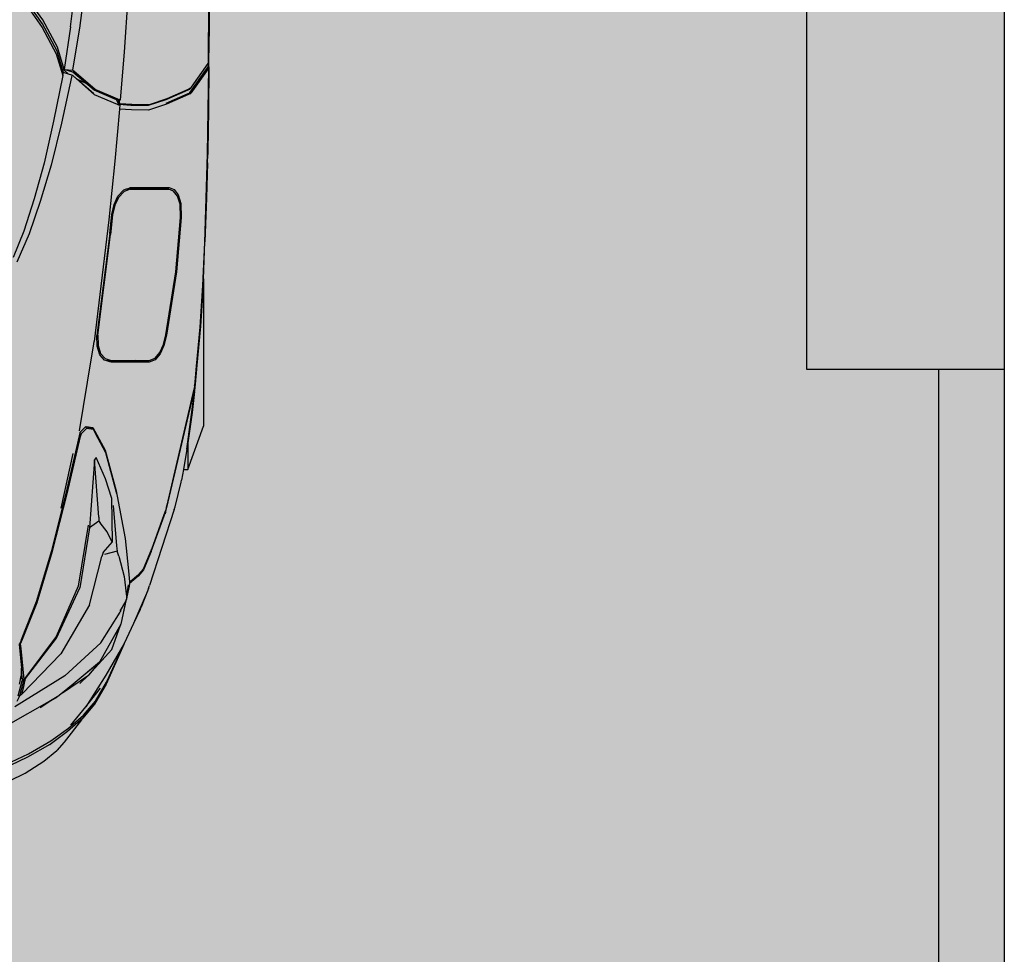
# Model space of a CAD drawing. Units: inches. Extents: x 1884 to 2398, y 474 to 1488.
# Tile 22 of 39: x 2352 to 2397, y 577 to 620. Entities that reach past the tile are written whole.
import ezdxf

# ---------------------------------------------------------------- set-up
doc = ezdxf.new("R2010")
doc.units = ezdxf.units.IN
doc.header["$MEASUREMENT"] = 0
doc.layers.get('0').update_dxf_attribs({"color": 250})
for name, color, linetype, lineweight in [('A-ANNO-DIMS', 2, 'Continuous', 18), ('A-WALL-PATT', 250, 'Continuous', 13), ('C-PROP', 7, 'Continuous', 30), ('C-VEHI', 8, 'Continuous', 18)]:
    doc.layers.add(name, color=color, linetype=linetype, lineweight=lineweight)
doc.layers.add('Edges', color=250, linetype='Continuous')
doc.layers.add('L-PVMT-PATT', color=9, linetype='Continuous', lineweight=13, true_color=0xc7c8ca)
doc.styles.get("Standard").update_dxf_attribs({"font": 'arial.ttf'})
doc.dimstyles.get("Standard").update_dxf_attribs({"dimtxt": 7, "dimasz": 0.18, "dimexe": 0.18, "dimexo": 0.0625, "dimgap": 0.09, "dimtad": 0, "dimtih": 1, "dimtoh": 1, "dimzin": 0, "dimdsep": 46, "dimlunit": 3, "dimtxsty": 'Standard', "dimcen": 0.09, "dimadec": 0, "dimazin": 0, "dimtfac": 1, "dimtofl": 0, "dimtmove": 0, "dimatfit": 3, "dimfxl": 1, "dimtolj": 1, "dimtzin": 0, "dimarcsym": 0})

# ---------------------------------------------------------------- blocks, each defined once
blk = doc.blocks.new('Nissan Qashqai pl')
at = {"layer": 'Edges'}
for p, q in [((10.6151, 12.8159), (10.6644, 12.8162)), ((10.6176, 12.8164), (10.6651, 12.8167)), ((10.6644, 12.8162), (10.7078, 12.8159)), ((10.6651, 12.8167), (10.666, 12.8167)), ((10.666, 12.8167), (10.677, 12.8167)), ((10.6729, 12.8157), (10.7082, 12.8156)), ((10.6809, 12.8167), (10.677, 12.8167)), ((10.7128, 12.8166), (10.6809, 12.8167)), ((10.7078, 12.8159), (10.7083, 12.8156)), ((10.7082, 12.8156), (10.7078, 12.8159)), ((10.7085, 12.8153), (10.7082, 12.8156)), ((10.7082, 12.8156), (10.7083, 12.8156)), ((10.7083, 12.8156), (10.7087, 12.8153)), ((10.7083, 12.8156), (10.7125, 12.8156)), ((10.7087, 12.8153), (10.7363, 12.7959)), ((10.7139, 12.8164), (10.7125, 12.8156)), ((10.7137, 12.8148), (10.7125, 12.8156)), ((10.7128, 12.8166), (10.7625, 12.8161)), ((10.7128, 12.8166), (10.724, 12.8166)), ((10.7137, 12.8148), (10.7138, 12.8147)), ((10.7418, 12.7947), (10.7138, 12.8147)), ((10.7139, 12.8164), (10.7148, 12.8157)), ((10.7628, 12.8158), (10.7139, 12.8164)), ((10.7148, 12.8157), (10.7429, 12.7956)), ((10.7685, 12.8161), (10.724, 12.8166)), ((10.7625, 12.8161), (10.7628, 12.8161)), ((10.7628, 12.8161), (10.8099, 12.8152)), ((10.8131, 12.8149), (10.7628, 12.8158)), ((10.7688, 12.8161), (10.7685, 12.8161)), ((10.8099, 12.8152), (10.7688, 12.8161)), ((10.8099, 12.8152), (10.8131, 12.8152)), ((10.8134, 12.8152), (10.8131, 12.8152)), ((10.8644, 12.8135), (10.8131, 12.8149)), ((10.8134, 12.8152), (10.8142, 12.8152)), ((10.8142, 12.8152), (10.8142, 12.8152)), ((10.8237, 12.8149), (10.8142, 12.8152)), ((10.8237, 12.8149), (10.864, 12.8138)), ((10.8596, 12.8138), (10.8589, 12.8138)), ((10.8642, 12.8136), (10.8596, 12.8138)), ((10.864, 12.8138), (10.8642, 12.8138)), ((10.8642, 12.8138), (10.9152, 12.812)), ((10.9158, 12.8118), (10.8644, 12.8135)), ((10.9577, 12.8101), (10.9152, 12.812)), ((10.9657, 12.8095), (10.9158, 12.8118)), ((10.9577, 12.8101), (10.9649, 12.8097)), ((10.9577, 12.8101), (11.1283, 12.8101)), ((10.9649, 12.8097), (11.0127, 12.8067)), ((11.0138, 12.8064), (10.9657, 12.8095)), ((11.0127, 12.8067), (11.0576, 12.8026)), ((11.1783, 12.7921), (11.1283, 12.8101)), ((10.7363, 12.7959), (10.7376, 12.795)), ((10.7432, 12.7954), (10.7426, 12.7954)), ((10.7429, 12.7956), (10.7432, 12.7954)), ((10.7441, 12.7954), (10.7432, 12.7954)), ((10.7432, 12.7954), (10.744, 12.7948)), ((11.059, 12.8023), (11.0138, 12.8064)), ((11.0576, 12.8026), (11.0798, 12.8008)), ((11.0768, 12.8008), (11.059, 12.8023)), ((11.0811, 12.8004), (11.0768, 12.8008)), ((11.0798, 12.8008), (11.0872, 12.7999)), ((11.0827, 12.8001), (11.0811, 12.8004)), ((11.0827, 12.8001), (11.0813, 12.7998)), ((11.0836, 12.8002), (11.0827, 12.8001)), ((11.0856, 12.7994), (11.0827, 12.8001)), ((11.0872, 12.7999), (11.0836, 12.8002)), ((11.0836, 12.8002), (11.0882, 12.7992)), ((11.2196, 12.7681), (11.0856, 12.7994)), ((11.0883, 12.7998), (11.0872, 12.7999)), ((11.0882, 12.7992), (11.2222, 12.7676)), ((11.0883, 12.7998), (11.1123, 12.797)), ((11.1147, 12.7965), (11.0883, 12.7998)), ((11.1123, 12.797), (11.1475, 12.7921)), ((11.1547, 12.791), (11.1147, 12.7965)), ((10.7387, 12.794), (10.7376, 12.795)), ((10.7376, 12.795), (10.7378, 12.7946)), ((10.7378, 12.7946), (10.7379, 12.7945)), ((10.7378, 12.7946), (10.7385, 12.7932)), ((10.7385, 12.7932), (10.7497, 12.7679)), ((10.7387, 12.794), (10.7396, 12.7922)), ((10.7396, 12.7922), (10.7507, 12.7669)), ((10.743, 12.7939), (10.7418, 12.7947)), ((10.7434, 12.793), (10.743, 12.7939)), ((10.7437, 12.7921), (10.7434, 12.793)), ((10.7438, 12.7921), (10.7437, 12.7921)), ((10.7438, 12.7921), (10.7549, 12.7666)), ((10.744, 12.7948), (10.7448, 12.793)), ((10.7448, 12.793), (10.7559, 12.7674)), ((10.8607, 12.7808), (10.8708, 12.7841)), ((10.8708, 12.7841), (10.8869, 12.7844)), ((10.8869, 12.7844), (10.9499, 12.7789)), ((11.1475, 12.7921), (11.1525, 12.7914)), ((11.1475, 12.7921), (11.1783, 12.7921)), ((11.1525, 12.7914), (11.1547, 12.791)), ((11.1547, 12.791), (11.1783, 12.787)), ((11.1783, 12.787), (11.1783, 12.7921)), ((11.1783, 12.787), (11.1906, 12.7849)), ((11.1906, 12.7849), (11.1909, 12.7849)), ((11.193, 12.7845), (11.1909, 12.7849)), ((11.2215, 12.7775), (11.193, 12.7845)), ((10.8523, 12.7704), (10.8546, 12.7762)), ((10.8565, 12.7757), (10.8543, 12.7702)), ((10.8546, 12.7762), (10.8607, 12.7808)), ((10.8622, 12.7801), (10.8565, 12.7757)), ((10.8716, 12.7832), (10.8622, 12.7801)), ((10.887, 12.7835), (10.8716, 12.7832)), ((10.9498, 12.7781), (10.887, 12.7835)), ((11.0226, 12.7668), (10.9498, 12.7781)), ((10.9499, 12.7789), (11.0229, 12.7676)), ((11.2247, 12.7764), (11.2215, 12.7775)), ((11.2247, 12.7764), (11.3124, 12.7479)), ((10.7497, 12.7679), (10.7565, 12.7473)), ((10.7507, 12.7669), (10.7575, 12.7462)), ((10.7559, 12.7674), (10.7626, 12.7467)), ((10.8523, 12.7255), (10.8523, 12.7704)), ((10.8543, 12.7702), (10.8538, 12.753)), ((10.8543, 12.7255), (10.8543, 12.7702)), ((11.0339, 12.7639), (11.0226, 12.7668)), ((11.0229, 12.7676), (11.0348, 12.7645)), ((11.0429, 12.7597), (11.0339, 12.7639)), ((11.0348, 12.7645), (11.0444, 12.7601)), ((11.2247, 12.767), (11.2163, 12.7689)), ((11.22, 12.768), (11.2196, 12.7681)), ((11.2247, 12.767), (11.22, 12.768)), ((11.2222, 12.7676), (11.2271, 12.7664)), ((11.2253, 12.7668), (11.2247, 12.767)), ((11.2304, 12.7649), (11.2253, 12.7668)), ((11.2253, 12.7668), (11.2271, 12.7664)), ((11.2271, 12.7664), (11.2296, 12.7658)), ((11.2271, 12.7664), (11.2277, 12.7662)), ((11.2277, 12.7662), (11.2296, 12.7658)), ((11.2732, 12.7496), (11.2277, 12.7662)), ((11.2704, 12.7504), (11.2304, 12.7649)), ((10.8528, 12.7503), (10.8535, 12.7521)), ((10.8528, 12.742), (10.8528, 12.7503)), ((10.8535, 12.7521), (10.8538, 12.753)), ((10.8538, 12.7521), (10.8535, 12.7521)), ((10.8538, 12.753), (10.8538, 12.7521)), ((10.8538, 12.7521), (10.8538, 12.7502)), ((10.8538, 12.7502), (10.8538, 12.742)), ((11.0497, 12.7542), (11.0429, 12.7597)), ((11.0444, 12.7601), (11.0516, 12.7542)), ((11.0523, 12.7475), (11.0497, 12.7542)), ((11.0516, 12.7542), (11.0543, 12.7473)), ((11.2702, 12.7507), (11.2704, 12.7504)), ((11.2704, 12.7506), (11.2707, 12.7503)), ((11.2707, 12.7503), (11.2704, 12.7504)), ((11.2719, 12.7498), (11.2707, 12.7503)), ((11.2934, 12.741), (11.2719, 12.7498)), ((10.7565, 12.7473), (10.7563, 12.7273)), ((10.7575, 12.7462), (10.7572, 12.7263)), ((10.7626, 12.7467), (10.7623, 12.7269)), ((10.8528, 12.742), (10.8538, 12.742)), ((10.8528, 12.7419), (10.8528, 12.742)), ((10.8538, 12.7419), (10.8528, 12.7419)), ((10.8528, 12.7242), (10.8528, 12.7419)), ((10.8538, 12.742), (10.8538, 12.7419)), ((10.8538, 12.7214), (10.8538, 12.7419)), ((11.0528, 12.73), (11.0523, 12.7475)), ((11.0523, 12.7312), (11.0523, 12.7475)), ((11.0543, 12.7473), (11.0543, 12.7035)), ((11.2732, 12.7496), (11.2946, 12.7409)), ((11.3, 12.735), (11.2934, 12.741)), ((11.2946, 12.7409), (11.3018, 12.7346)), ((11.3161, 12.7467), (11.3124, 12.7479)), ((11.3161, 12.7467), (11.3376, 12.7381)), ((11.3192, 12.7454), (11.3566, 12.7294)), ((10.7563, 12.7273), (10.7553, 12.7134)), ((11.0523, 12.7312), (11.0528, 12.73)), ((11.0523, 12.7287), (11.0523, 12.7312)), ((11.0528, 12.7274), (11.0523, 12.7287)), ((11.0523, 12.7037), (11.0523, 12.7287)), ((11.0528, 12.7274), (11.0528, 12.73)), ((11.0528, 12.73), (11.0538, 12.7273)), ((11.0528, 12.7274), (11.0528, 12.6985)), ((11.0538, 12.7273), (11.0538, 12.7018)), ((11.3081, 12.7253), (11.3, 12.735)), ((11.3018, 12.7346), (11.3103, 12.7249)), ((11.3405, 12.7369), (11.3376, 12.7381)), ((11.3405, 12.7369), (11.3566, 12.7294)), ((11.3566, 12.7294), (11.3796, 12.7187)), ((10.6318, 12.7228), (10.6955, 12.7184)), ((10.6955, 12.7184), (10.7509, 12.714)), ((10.7572, 12.7263), (10.7563, 12.7126)), ((10.7623, 12.7269), (10.7615, 12.7131)), ((10.8528, 12.7242), (10.8523, 12.7255)), ((10.8538, 12.7214), (10.8528, 12.7242)), ((10.855, 12.7181), (10.8538, 12.7214)), ((10.8543, 12.7255), (10.8569, 12.7184)), ((10.8622, 12.7114), (10.855, 12.7181)), ((10.8569, 12.7184), (10.8637, 12.712)), ((11.2091, 12.7103), (11.2583, 12.7196)), ((11.2583, 12.7196), (11.2956, 12.7234)), ((11.2787, 12.7123), (11.3022, 12.7186)), ((11.2956, 12.7234), (11.3085, 12.7247)), ((11.3022, 12.7186), (11.3252, 12.7213)), ((11.3086, 12.7247), (11.3081, 12.7253)), ((11.3081, 12.7253), (11.3087, 12.7247)), ((11.3085, 12.7247), (11.3086, 12.7247)), ((11.3086, 12.7247), (11.3087, 12.7247)), ((11.3087, 12.7247), (11.3103, 12.7249)), ((11.3103, 12.7249), (11.3103, 12.7249)), ((11.3103, 12.7249), (11.3106, 12.7249)), ((11.3106, 12.7249), (11.314, 12.7238)), ((11.317, 12.7227), (11.3119, 12.7236)), ((11.3132, 12.7243), (11.3256, 12.7215)), ((11.314, 12.7238), (11.317, 12.7227)), ((11.314, 12.7238), (11.3242, 12.7216)), ((11.3242, 12.7216), (11.317, 12.7227)), ((11.3198, 12.7211), (11.3252, 12.7213)), ((11.3242, 12.7216), (11.3256, 12.7215)), ((11.3252, 12.7213), (11.3283, 12.7214)), ((11.3256, 12.7215), (11.3283, 12.7214)), ((11.3283, 12.7214), (11.3297, 12.7206)), ((11.3297, 12.7206), (11.3446, 12.7173)), ((11.3297, 12.7206), (11.3302, 12.7203)), ((11.3302, 12.7203), (11.3446, 12.7173)), ((11.3302, 12.7203), (11.3394, 12.7152)), ((11.3446, 12.7173), (11.3571, 12.7146)), ((11.3796, 12.7187), (11.4164, 12.6974)), ((11.3796, 12.7187), (11.3807, 12.7182)), ((11.3807, 12.7182), (11.4267, 12.6979)), ((11.4228, 12.6989), (11.3807, 12.7182)), ((10.7501, 12.7114), (10.7387, 12.6849)), ((10.7507, 12.7098), (10.7397, 12.684)), ((10.7563, 12.7109), (10.7449, 12.6843)), ((10.7507, 12.7132), (10.7501, 12.7114)), ((10.7506, 12.7111), (10.7507, 12.7132)), ((10.7507, 12.7132), (10.7509, 12.714)), ((10.751, 12.7132), (10.7507, 12.7132)), ((10.7511, 12.7107), (10.7507, 12.7098)), ((10.7524, 12.7106), (10.7507, 12.7098)), ((10.7522, 12.7131), (10.7509, 12.714)), ((10.7516, 12.7131), (10.7509, 12.714)), ((10.7519, 12.7128), (10.7511, 12.7107)), ((10.7522, 12.7131), (10.7516, 12.7131)), ((10.7519, 12.7128), (10.7516, 12.7131)), ((10.7526, 12.7124), (10.7519, 12.7128)), ((10.7553, 12.7134), (10.7522, 12.7131)), ((10.7524, 12.7106), (10.7526, 12.7124)), ((10.7556, 12.7122), (10.7524, 12.7106)), ((10.7526, 12.7124), (10.7526, 12.7127)), ((10.7532, 12.712), (10.7526, 12.7124)), ((10.7556, 12.7122), (10.7532, 12.712)), ((10.7561, 12.7125), (10.7556, 12.7122)), ((10.7561, 12.7125), (10.7563, 12.7126)), ((10.7563, 12.7125), (10.7561, 12.7125)), ((10.7563, 12.7123), (10.7561, 12.7123)), ((10.7563, 12.7126), (10.7573, 12.7135)), ((10.7563, 12.7126), (10.7563, 12.7125)), ((10.7569, 12.7125), (10.7563, 12.7109)), ((10.7569, 12.7125), (10.7563, 12.7125)), ((10.7563, 12.7125), (10.7563, 12.7123)), ((10.7573, 12.7135), (10.7569, 12.7125)), ((10.7573, 12.7135), (10.7604, 12.7132)), ((10.7604, 12.7132), (10.7615, 12.7131)), ((10.7615, 12.7131), (10.8218, 12.7077)), ((10.8218, 12.7077), (10.8896, 12.7008)), ((10.8718, 12.7068), (10.8622, 12.7114)), ((10.8637, 12.712), (10.8727, 12.7077)), ((10.8836, 12.7041), (10.8718, 12.7068)), ((10.8727, 12.7077), (10.8839, 12.7051)), ((10.8839, 12.7051), (10.9067, 12.7029)), ((11.156, 12.6966), (11.203, 12.7093)), ((11.1589, 12.6971), (11.2062, 12.7098)), ((11.2121, 12.7043), (11.189, 12.6968)), ((11.203, 12.7093), (11.2091, 12.7103)), ((11.2062, 12.7098), (11.2091, 12.7103)), ((11.2622, 12.7051), (11.2121, 12.7043)), ((11.2199, 12.706), (11.2666, 12.7097)), ((11.2622, 12.7051), (11.2601, 12.7037)), ((11.2743, 12.6942), (11.2622, 12.7051)), ((11.2666, 12.7097), (11.2729, 12.7104)), ((11.2787, 12.7123), (11.2729, 12.7104)), ((11.2729, 12.7104), (11.2766, 12.6957)), ((11.3394, 12.7152), (11.3434, 12.7138)), ((11.3394, 12.7152), (11.342, 12.7137)), ((11.379, 12.6915), (11.3434, 12.7138)), ((11.3583, 12.7142), (11.3571, 12.7146)), ((11.3571, 12.7146), (11.3821, 12.7008)), ((11.3583, 12.7142), (11.3821, 12.7008)), ((11.3864, 12.7044), (11.3583, 12.7142)), ((11.4163, 12.6775), (11.3864, 12.7044)), ((10.9054, 12.702), (10.8836, 12.7041)), ((10.8896, 12.7008), (11.0304, 12.6838)), ((10.9054, 12.702), (11.0232, 12.6871)), ((11.0231, 12.6882), (10.9067, 12.7029)), ((11.0443, 12.6911), (11.0501, 12.6964)), ((11.052, 12.6958), (11.0458, 12.6903)), ((11.0501, 12.6964), (11.0523, 12.7037)), ((11.0528, 12.6985), (11.052, 12.6958)), ((11.0538, 12.7018), (11.0528, 12.6985)), ((11.0543, 12.7035), (11.0538, 12.7018)), ((11.1298, 12.6823), (11.156, 12.6966)), ((11.1365, 12.6851), (11.1589, 12.6971)), ((11.189, 12.6968), (11.1644, 12.6862)), ((11.2505, 12.6987), (11.2401, 12.6908)), ((11.2601, 12.7037), (11.2505, 12.6987)), ((11.2743, 12.6942), (11.2791, 12.6927)), ((11.3821, 12.7008), (11.4014, 12.69)), ((11.4164, 12.6974), (11.4531, 12.6744)), ((11.4243, 12.6982), (11.4228, 12.6989)), ((11.4464, 12.6853), (11.4243, 12.6982)), ((11.4267, 12.6979), (11.4498, 12.6844)), ((10.7387, 12.6849), (10.7177, 12.6604)), ((10.7449, 12.6843), (10.7232, 12.6594)), ((10.7438, 12.6836), (10.7265, 12.6635)), ((10.7397, 12.684), (10.7334, 12.6766)), ((11.0231, 12.6882), (11.035, 12.6883)), ((11.0358, 12.6872), (11.0232, 12.6871)), ((11.0357, 12.6829), (11.0304, 12.6838)), ((11.035, 12.6883), (11.0443, 12.6911)), ((11.0491, 12.6807), (11.0357, 12.6829)), ((11.0458, 12.6903), (11.0358, 12.6872)), ((11.1285, 12.6745), (11.1298, 12.6823)), ((11.1306, 12.6752), (11.1319, 12.6827)), ((11.1319, 12.6827), (11.1306, 12.6812)), ((11.1319, 12.6827), (11.1365, 12.6851)), ((11.1644, 12.6862), (11.1672, 12.6844)), ((11.2337, 12.6892), (11.1672, 12.6844)), ((11.1672, 12.6844), (11.2459, 12.6785)), ((11.2337, 12.6892), (11.2382, 12.6892)), ((11.2382, 12.6892), (11.2401, 12.6908)), ((11.2382, 12.6892), (11.2459, 12.6785)), ((11.335, 12.6786), (11.2791, 12.6927)), ((11.379, 12.6915), (11.417, 12.6499)), ((11.4014, 12.69), (11.4022, 12.6894)), ((11.4014, 12.69), (11.4265, 12.6594)), ((11.4022, 12.6894), (11.4163, 12.6775)), ((11.4022, 12.6894), (11.4265, 12.6594)), ((11.4531, 12.6744), (11.4314, 12.6911)), ((11.4624, 12.6717), (11.4464, 12.6853)), ((11.4498, 12.6844), (11.4662, 12.6706)), ((11.4681, 12.6691), (11.4498, 12.6844)), ((10.6678, 12.6672), (10.6152, 12.674)), ((10.7334, 12.6766), (10.7186, 12.6593)), ((10.7265, 12.6635), (10.7316, 12.6741)), ((11.0449, 12.6812), (11.0448, 12.6812)), ((11.0492, 12.6807), (11.0491, 12.6807)), ((11.1336, 12.667), (11.0492, 12.6807)), ((11.1293, 12.6736), (11.1285, 12.6745)), ((11.1306, 12.6812), (11.1293, 12.6736)), ((11.1353, 12.6677), (11.1293, 12.6736)), ((11.1347, 12.671), (11.1306, 12.6752)), ((11.1366, 12.6691), (11.1347, 12.671)), ((11.2428, 12.6769), (11.3132, 12.6652)), ((11.2459, 12.6785), (11.3153, 12.6672)), ((11.335, 12.6786), (11.3915, 12.6453)), ((11.4366, 12.6471), (11.4163, 12.6775)), ((11.4163, 12.6775), (11.4259, 12.6674)), ((11.4742, 12.6567), (11.4531, 12.6744)), ((11.4774, 12.6543), (11.4624, 12.6717)), ((11.4662, 12.6706), (11.4815, 12.6531)), ((10.6664, 12.6566), (10.6144, 12.6629)), ((10.7137, 12.6595), (10.6678, 12.6672)), ((10.7165, 12.6591), (10.7137, 12.6595)), ((10.7186, 12.6593), (10.7155, 12.649)), ((10.7155, 12.649), (10.7165, 12.6591)), ((10.7177, 12.6604), (10.7165, 12.6591)), ((10.7232, 12.6594), (10.7221, 12.6581)), ((10.7221, 12.6581), (10.7224, 12.6587)), ((10.7265, 12.6635), (10.7224, 12.6587)), ((11.1358, 12.6676), (11.1353, 12.6677)), ((11.1358, 12.6676), (11.1366, 12.6691)), ((11.148, 12.665), (11.1358, 12.6676)), ((11.1401, 12.6682), (11.1366, 12.6691)), ((11.2066, 12.6527), (11.1401, 12.6682)), ((11.2063, 12.6515), (11.148, 12.665)), ((11.2232, 12.6458), (11.1598, 12.6594)), ((11.3132, 12.6652), (11.3715, 12.6398)), ((11.3733, 12.6404), (11.3153, 12.6672)), ((11.4265, 12.6594), (11.4366, 12.6471)), ((11.4681, 12.6691), (11.4936, 12.6491)), ((10.6664, 12.6566), (10.7155, 12.649)), ((10.7155, 12.649), (10.69, 12.6414)), ((10.7155, 12.6473), (10.6943, 12.641)), ((10.6976, 12.6401), (10.7228, 12.6477)), ((10.7209, 12.654), (10.7155, 12.6485)), ((10.7155, 12.649), (10.7155, 12.6485)), ((10.7155, 12.6485), (10.7155, 12.6473)), ((10.7192, 12.6484), (10.7155, 12.6473)), ((10.7209, 12.654), (10.7192, 12.6484)), ((10.7228, 12.6477), (10.7192, 12.6484)), ((10.7221, 12.6581), (10.7209, 12.654)), ((10.7221, 12.6581), (10.7247, 12.6575)), ((10.7228, 12.6477), (10.7754, 12.637)), ((10.7247, 12.6575), (10.7776, 12.646)), ((11.272, 12.6349), (11.2063, 12.6515)), ((11.2728, 12.6357), (11.2066, 12.6527)), ((11.417, 12.6499), (11.4529, 12.5922)), ((11.4924, 12.6339), (11.4774, 12.6543)), ((11.4815, 12.6531), (11.4963, 12.6328)), ((11.4936, 12.6491), (11.5033, 12.6408)), ((10.69, 12.6414), (10.6583, 12.6245)), ((10.6943, 12.641), (10.6627, 12.6241)), ((10.6671, 12.6238), (10.6976, 12.6401)), ((10.7754, 12.637), (10.8239, 12.6261)), ((10.7776, 12.646), (10.8264, 12.6341)), ((11.3715, 12.6398), (11.4177, 12.6052)), ((11.4203, 12.6044), (11.3733, 12.6404)), ((11.3915, 12.6453), (11.4381, 12.6002)), ((11.4366, 12.6471), (11.4408, 12.6419)), ((11.4408, 12.6419), (11.4411, 12.6414)), ((11.4411, 12.6414), (11.4411, 12.6414)), ((11.4414, 12.6409), (11.4411, 12.6414)), ((11.4414, 12.6409), (11.447, 12.6315)), ((11.4455, 12.6336), (11.4414, 12.6409)), ((11.5158, 12.6256), (11.5033, 12.6408)), ((10.6583, 12.6245), (10.6215, 12.5986)), ((10.8239, 12.6261), (10.8653, 12.6144)), ((10.8264, 12.6341), (10.8682, 12.6216)), ((11.3311, 12.6172), (11.272, 12.6349)), ((11.3323, 12.6178), (11.2728, 12.6357)), ((11.447, 12.6315), (11.4455, 12.6336)), ((11.4455, 12.6336), (11.4462, 12.6324)), ((11.447, 12.6315), (11.4462, 12.6324)), ((11.4732, 12.585), (11.4462, 12.6324)), ((11.447, 12.6315), (11.447, 12.6314)), ((11.4536, 12.6215), (11.447, 12.6314)), ((11.5074, 12.608), (11.4924, 12.6339)), ((11.4964, 12.6326), (11.4963, 12.6328)), ((11.4964, 12.6326), (11.5113, 12.6069)), ((11.5295, 12.6041), (11.5158, 12.6256)), ((10.6627, 12.6241), (10.6261, 12.5984)), ((10.6306, 12.5982), (10.6671, 12.6238)), ((10.8653, 12.6144), (10.9026, 12.6025)), ((10.8682, 12.6216), (10.9059, 12.6087)), ((11.3751, 12.5999), (11.3311, 12.6172)), ((11.3747, 12.6011), (11.3323, 12.6178)), ((10.9026, 12.6025), (10.933, 12.5901)), ((10.9059, 12.6087), (10.9384, 12.5945)), ((11.4212, 12.603), (11.3853, 12.5993)), ((11.4177, 12.6052), (11.4193, 12.6042)), ((11.4192, 12.6045), (11.4194, 12.6042)), ((11.4194, 12.6042), (11.4193, 12.6042)), ((11.4193, 12.6042), (11.4196, 12.604)), ((11.4194, 12.6042), (11.4196, 12.604)), ((11.4196, 12.6042), (11.4194, 12.6042)), ((11.4196, 12.604), (11.4201, 12.6036)), ((11.4198, 12.6041), (11.4201, 12.6036)), ((11.4201, 12.6036), (11.4212, 12.603)), ((11.4292, 12.6024), (11.4203, 12.6044)), ((11.4229, 12.6025), (11.4203, 12.6044)), ((11.4212, 12.603), (11.4215, 12.601)), ((11.4218, 12.6028), (11.4212, 12.603)), ((11.4222, 12.6029), (11.4218, 12.6028)), ((11.4229, 12.6025), (11.4218, 12.6028)), ((11.4315, 12.6002), (11.4229, 12.6025)), ((11.423, 12.6006), (11.4229, 12.6025)), ((11.4381, 12.6002), (11.4292, 12.6024)), ((11.5165, 12.5882), (11.5074, 12.608)), ((11.5113, 12.6068), (11.5113, 12.6069)), ((11.5113, 12.6068), (11.5206, 12.5869)), ((11.5384, 12.5859), (11.5295, 12.6041)), ((11.38, 12.5988), (11.3747, 12.6011)), ((11.3751, 12.5999), (11.3762, 12.5999)), ((11.3752, 12.5998), (11.3751, 12.5999)), ((11.3763, 12.5998), (11.3752, 12.5998)), ((11.3764, 12.5993), (11.3752, 12.5998)), ((11.3792, 12.5982), (11.3764, 12.5993)), ((11.3792, 12.5982), (11.3793, 12.5979)), ((11.3792, 12.5982), (11.3804, 12.5972)), ((11.3853, 12.5993), (11.38, 12.5988)), ((11.3804, 12.5972), (11.4082, 12.5998)), ((11.409, 12.5999), (11.4082, 12.5998)), ((11.4164, 12.5998), (11.4082, 12.5998)), ((11.4152, 12.6004), (11.409, 12.5999)), ((11.409, 12.5999), (11.4163, 12.5999)), ((11.4173, 12.6006), (11.4152, 12.6004)), ((11.4163, 12.5999), (11.4152, 12.6004)), ((11.4163, 12.5999), (11.4186, 12.5999)), ((11.4164, 12.5998), (11.4163, 12.5999)), ((11.4181, 12.5998), (11.4164, 12.5998)), ((11.4169, 12.5996), (11.4164, 12.5998)), ((11.4252, 12.598), (11.4169, 12.5996)), ((11.4176, 12.6007), (11.4173, 12.6006)), ((11.418, 12.6006), (11.4173, 12.6006)), ((11.4215, 12.601), (11.4176, 12.6007)), ((11.418, 12.6006), (11.4176, 12.6007)), ((11.4204, 12.6002), (11.418, 12.6006)), ((11.4194, 12.6), (11.418, 12.6006)), ((11.4215, 12.601), (11.4219, 12.6009)), ((11.4219, 12.6009), (11.4222, 12.6005)), ((11.4219, 12.6009), (11.4224, 12.6008)), ((11.4224, 12.6008), (11.4226, 12.6006)), ((11.4224, 12.6008), (11.423, 12.6006)), ((11.44, 12.5959), (11.423, 12.6006)), ((11.4266, 12.5977), (11.4252, 12.598)), ((11.4403, 12.5978), (11.4315, 12.6002)), ((11.4381, 12.6002), (11.4403, 12.5978)), ((11.4403, 12.5978), (11.44, 12.5959)), ((11.4462, 12.5947), (11.4403, 12.5978))]:
    blk.add_line(p, q, dxfattribs=at)
blk = doc.blocks.new('car')
blk.add_blockref('Nissan Qashqai pl', (-9.7433, -11.9151))
blk = doc.blocks.new('carr')
blk.add_blockref('car', (0.5124, -0.007))
blk = doc.blocks.new('*D49')
at = {"layer": 'A-ANNO-DIMS', "color": 0, "lineweight": -2, "transparency": 16777216}
for p, q in [((2318.409, 987.716), (2318.409, 484.005)), ((2340.409, 987.716), (2340.409, 484.005)), ((2318.589, 484.185), (2340.229, 484.185)), ((2340.409, 484.185), (2340.589, 484.185))]:
    blk.add_line(p, q, dxfattribs=at)
at = {"layer": 'A-ANNO-DIMS', "color": 0, "lineweight": 100, "transparency": 16777216}
for points in [[(2318.589, 484.215), (2318.589, 484.155), (2318.409, 484.185)], [(2340.229, 484.215), (2340.229, 484.155), (2340.409, 484.185)]]:
    blk.add_solid(points, dxfattribs=at)
at = {"layer": 'Defpoints', "color": 0, "lineweight": 100, "transparency": 16777216}
for p in [(2318.409, 987.778), (2340.409, 987.778), (2340.409, 484.185)]:
    blk.add_point(p, dxfattribs=at)
at = {"layer": 'A-ANNO-DIMS', "color": 0, "transparency": 16777216, "insert": (2352.373, 484.185), "char_height": 7, "attachment_point": 5}
blk.add_mtext('\\A1;1\'-10"', dxfattribs=at)

msp = doc.modelspace()

# ---------------------------------------------------------------- hatches: boundary and pattern name
at = {"layer": 'A-WALL-PATT'}
h = msp.add_hatch(color=256, dxfattribs=at)
h.dxf.hatch_style = 1
h.paths.add_polyline_path([(2351.529, 837.963), (2342.529, 837.963), (2342.529, 813.478), (2351.529, 813.478)])
h.paths.add_polyline_path([(2351.529, 782.175), (2342.529, 782.175), (2342.529, 778.966), (2238.447, 778.966), (2238.447, 769.966), (2351.529, 769.966)])
h.paths.add_polyline_path([(2351.529, 914.773), (2342.529, 914.773), (2342.529, 901.966), (2222.529, 901.966), (2222.529, 908.236), (2213.529, 908.236), (2213.529, 901.966), (2198.529, 901.966), (2198.529, 892.966), (2198.529, 815.857), (2203.029, 815.857), (2203.029, 892.966), (2342.529, 892.966), (2342.529, 869.555), (2346.047, 869.555), (2351.529, 869.555), (2351.529, 880.385)])
h.paths.add_polyline_path([(2208.948, 778.966), (2203.029, 778.966), (2203.029, 782.647), (2198.529, 782.647), (2198.529, 779.109), (2193.526, 779.109), (2193.526, 769.966), (2198.529, 769.966), (2208.948, 769.966)])
h.paths.add_polyline_path([(2126.529, 815.801), (2117.529, 815.801), (2117.529, 676.183), (2126.529, 676.183), (2126.529, 769.966), (2132.515, 769.966), (2132.515, 778.664), (2126.529, 778.664)])
h.paths.add_polyline_path([(2135.996, 901.385), (2009.529, 901.385), (2009.529, 929.544), (2000.529, 929.544), (2000.529, 892.385), (2117.529, 892.385), (2117.529, 880.382), (2126.529, 880.382), (2126.529, 892.385), (2135.996, 892.385)])
h.paths.add_polyline_path([(2198.529, 901.385), (2185.2, 901.385), (2185.2, 892.385), (2198.529, 892.385), (2198.529, 892.966)])
h.paths.add_polyline_path([(1961.529, 892.385), (1965.143, 892.385), (1965.143, 901.385), (1952.529, 901.385), (1952.529, 604.13), (1961.529, 604.13), (1961.529, 631.385), (1988.002, 631.385), (1988.002, 640.385), (1961.529, 640.385)])
h.paths.add_polyline_path([(1955.529, 604.13), (1952.529, 604.13), (1952.529, 530.885), (2126.529, 530.885), (2126.529, 533.885), (1955.529, 533.885)])
h.paths.add_polyline_path([(2396.529, 604.13), (2393.529, 604.13), (2393.529, 533.885), (2126.529, 533.885), (2126.529, 530.885), (2396.529, 530.885)])
h.paths.add_polyline_path([(2396.529, 779.322), (2387.529, 779.322), (2387.529, 604.13), (2396.529, 604.13)])
at = {"layer": 'L-PVMT-PATT'}
h = msp.add_hatch(color=256, dxfattribs=at)
h.dxf.hatch_style = 1
h.paths.add_polyline_path([(2387.529, 769.966), (2351.529, 769.966), (2238.447, 769.966), (2238.447, 762.15), (2238.447, 754.445), (2126.529, 754.445), (2126.529, 676.183), (2134.868, 676.183), (2142.673, 676.183), (2142.673, 646.578), (2134.868, 646.578), (2126.529, 646.578), (2126.529, 640.17), (2387.529, 640.17)])
h.paths.add_polyline_path([(2387.529, 631.385), (2303.086, 631.385), (2303.086, 615.671), (2387.529, 615.671)])
h.paths.add_polyline_path([(2387.529, 640.17), (2126.529, 640.17), (2126.529, 631.385), (2387.529, 631.385)])
h.paths.add_polyline_path([(2393.529, 604.13), (2387.529, 604.13), (2387.529, 615.671), (2303.086, 615.671), (2303.086, 607.943), (2249.649, 607.943), (2126.529, 607.943), (2126.529, 533.885), (2393.529, 533.885)])
h.paths.add_polyline_path([(2257.825, 611.008), (2257.83, 611.337), (2257.915, 616.493), (2258.021, 621.805), (2258.146, 627.274), (2258.252, 631.385), (2126.529, 631.385), (2126.529, 611.008)])
h.paths.add_polyline_path([(2258.892, 611.285), (2258.888, 611.008), (2300.247, 611.008), (2300.247, 631.385), (2259.314, 631.385), (2259.206, 627.173), (2259.081, 621.72), (2258.976, 616.424)])

# ---------------------------------------------------------------- linework, layer by layer
at = {"layer": 'C-PROP'}
for p, q in [((2396.529, 1406.885), (2396.529, 530.885)), ((2387.529, 779.322), (2387.529, 604.13)), ((2387.529, 604.13), (2396.529, 604.13)), ((2393.529, 604.13), (2393.529, 533.885))]:
    msp.add_line(p, q, dxfattribs=at)

# ---------------------------------------------------------------- block references
at = {"layer": 'C-VEHI', "xscale": 39.37007874015748, "yscale": 39.37007874015748, "zscale": 39.37007874015748, "rotation": 270}
msp.add_blockref('carr', (2325.111, 676.232), dxfattribs=at)

# ---------------------------------------------------------------- dimensions: what is measured, and where the dimension line sits
at = {"layer": 'A-ANNO-DIMS'}
dim = msp.add_linear_dim(base=(2340.409, 484.185), p1=(2318.409, 987.778), p2=(2340.409, 987.778), dimstyle='Standard', override={"dimdec": 1, "dimlfac": 1, "dimrnd": 0, "dimzin": 1, "dimdsep": 46, "dimlunit": 4, "dimfrac": 2}, dxfattribs=at)
dim.commit()
dim.dimension.update_dxf_attribs({"geometry": '*D49', "text_midpoint": (2352.373, 484.185)})

doc.saveas('drawing.dxf')
